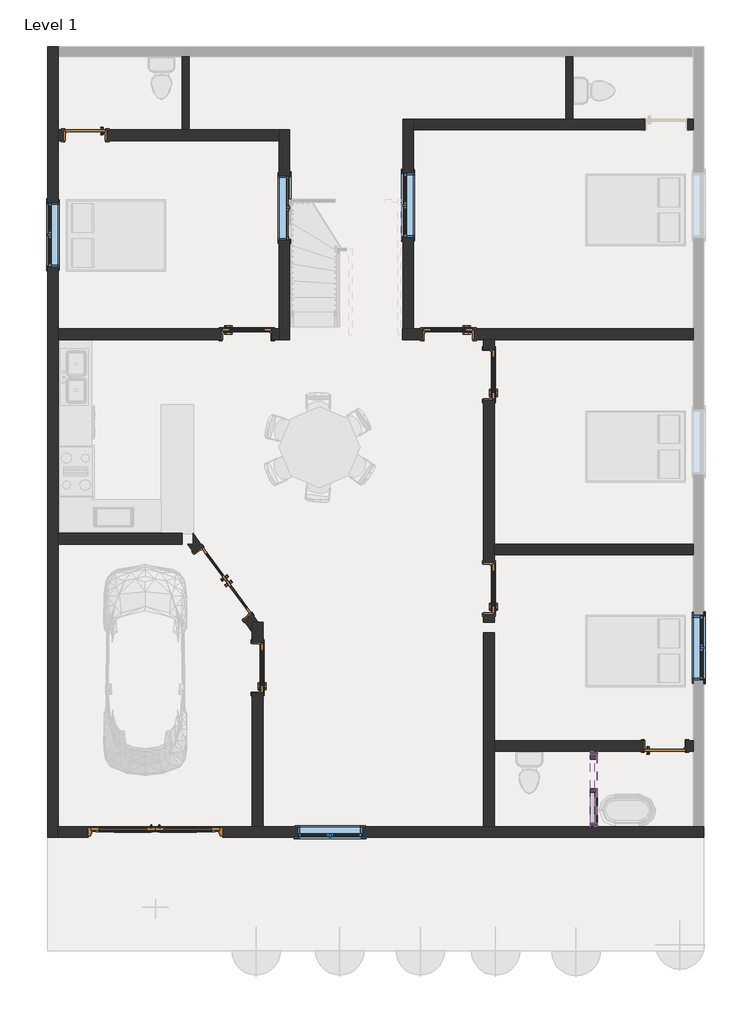
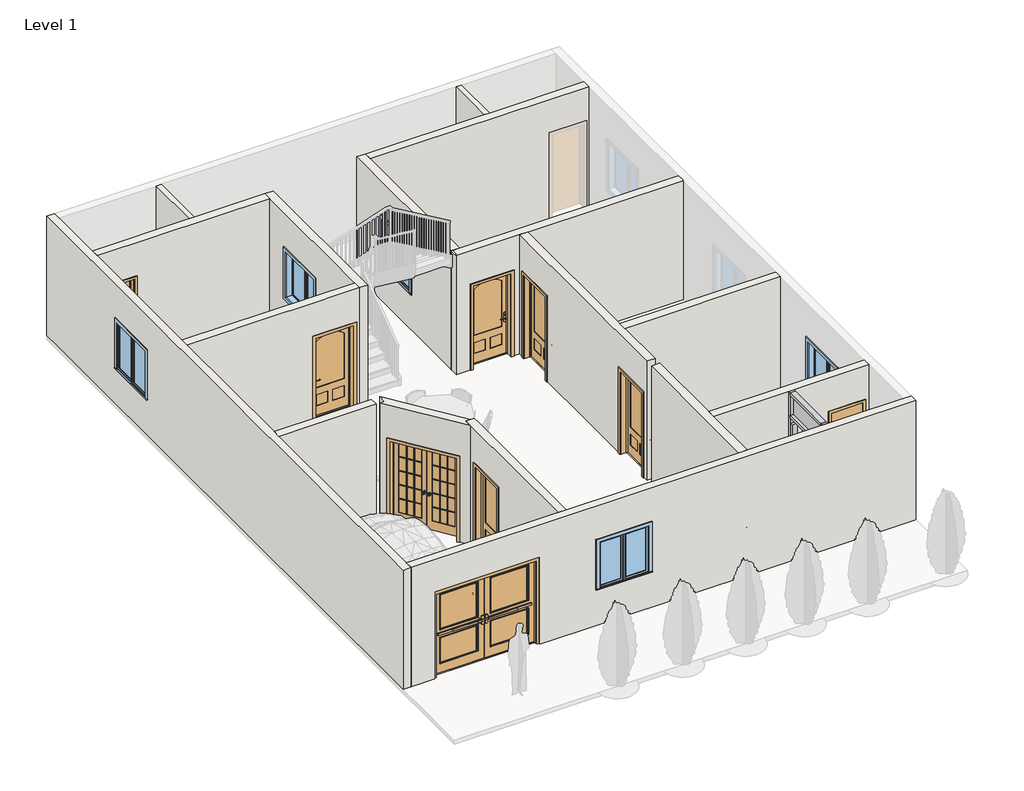
# One storey, part 1 of 3: 17 walls, 10 members, 9 doors, 5 windows, 2 plates.
"""IFC4 building model written with IfcOpenShell, lengths in millimetres."""

from ifc_helpers import new_model, si_unit, frame, origin, origin_with_axes, place, context, project, spatial, polyline, outline, extrude, faceted_brep, transform, mapped, element, save
from components import door_4a215221, door_9fdf8246, door_14451ac2, door_142f3e8c, door_1bf41894, door_15ec6cad, door_701f8457, member_ee409385, member_c8c2a2fa, member_ccee4eb0, member_cc169a76, member_860c46db, member_ba732fc4, member_623bfa76, member_547128e5, member_47bfaf8a, system_panel_glazed_bef2143c, system_panel_glazed_3ed2553b, window_0862ab64, window_d2c79e1c

model = new_model("IFC4")

# Units and contexts
model_context = context("Model", 3, world=origin())
ifc_project = project(units=[si_unit("LENGTHUNIT", "METRE", prefix="MILLI")], contexts=[model_context])

# Site, building, storey
site = spatial("IfcSite", under=ifc_project)
building = spatial("IfcBuilding", under=site)
storey = spatial("IfcBuildingStorey", under=building, Name="Level 1", Elevation=0.0)

# Doors
placement = place(None, origin())
door_shape = door_4a215221(model_context)
element("IfcDoor", 1, ObjectType="36\" x 84\"", at=placement, inside=storey, context=model_context, shape_type="MappedRepresentation", body=[
    mapped(door_shape, transform((5765.6625253, 2165.4527309, 0.0), x_axis=(0.0, -1.0, 0.0), y_axis=(1.0, 0.0, 0.0), z_axis=(0.0, 0.0, 1.0))),
])
element("IfcDoor", 2, ObjectType="36\" x 84\"", at=placement, inside=storey, context=model_context, shape_type="MappedRepresentation", body=[
    mapped(door_shape, transform((5765.6625253, -1873.1472691, 0.0), x_axis=(0.0, -1.0, 0.0), y_axis=(1.0, 0.0, 0.0), z_axis=(0.0, 0.0, 1.0))),
])
element("IfcDoor", 3, ObjectType="36\" x 84\"", at=placement, inside=storey, context=model_context, shape_type="MappedRepresentation", body=[
    mapped(door_shape, transform((4995.7250253, 2930.6277309, 0.0), x_axis=(1.0, 0.0, 0.0), y_axis=(0.0, 1.0, 0.0), z_axis=(0.0, 0.0, 1.0))),
])
element("IfcDoor", 4, ObjectType="36\" x 84\"", at=placement, inside=storey, context=model_context, shape_type="MappedRepresentation", body=[
    mapped(door_shape, transform((1392.1000253, -3371.7472691, 0.0), x_axis=(0.0, -1.0, 0.0), y_axis=(1.0, 0.0, 0.0), z_axis=(0.0, 0.0, 1.0))),
])
door_2_shape = door_9fdf8246(model_context)
element("IfcDoor", 5, ObjectType="36\" x 84\"", at=placement, inside=storey, context=model_context, shape_type="MappedRepresentation", body=[
    mapped(door_2_shape, transform((1185.7250253, 2930.6277309, 0.0), x_axis=(-1.0, 0.0, 0.0), y_axis=(0.0, -1.0, 0.0), z_axis=(0.0, 0.0, 1.0))),
])
door_3_shape = door_14451ac2(model_context)
door_4_shape = door_142f3e8c(model_context)
door_5_shape = door_1bf41894(model_context)
element("IfcDoor", 6, ObjectType="Door-Exterior-Double-Two_Lite : 96\" x 84\"", at=placement, inside=storey, context=model_context, shape_type="MappedRepresentation", body=[
    mapped(door_3_shape, transform((-541.4749747, -6476.8972691, 0.0), x_axis=(1.0, 0.0, 0.0), y_axis=(0.0, 1.0, 0.0), z_axis=(0.0, 0.0, 1.0))),
    mapped(door_4_shape, transform((-541.4749747, -6476.8972691, 0.0), x_axis=(1.0, 0.0, 0.0), y_axis=(0.0, 1.0, 0.0), z_axis=(0.0, 0.0, 1.0))),
    mapped(door_5_shape, transform((-541.4749747, -6476.8972691, 0.0), x_axis=(1.0, 0.0, 0.0), y_axis=(0.0, 1.0, 0.0), z_axis=(0.0, 0.0, 1.0))),
])
door_6_shape = door_15ec6cad(model_context)
element("IfcDoor", 7, ObjectType="Door-Interior-Double-Full Glass-Wood : 60\" x 84\"", at=placement, inside=storey, context=model_context, shape_type="MappedRepresentation", body=[
    mapped(door_6_shape, transform((739.9205393, -1775.5962656, 0.0), x_axis=(0.5914191036451608, -0.8063643369120156, 0.0), y_axis=(0.8063643369120156, 0.5914191036451608, 0.0), z_axis=(0.0, 0.0, 1.0))),
])
door_7_shape = door_701f8457(model_context)
element("IfcDoor", 8, ObjectType="Door-Interior-Single-Flush_Panel-Wood : 30\" x 84\"", at=placement, inside=storey, context=model_context, shape_type="MappedRepresentation", body=[
    mapped(door_7_shape, transform((-1867.0374747, 6689.8277309, 0.0), x_axis=(-1.0, 0.0, 0.0), y_axis=(0.0, -1.0, 0.0), z_axis=(0.0, 0.0, 1.0))),
])
element("IfcDoor", 9, ObjectType="Door-Interior-Single-Flush_Panel-Wood : 30\" x 84\"", at=placement, inside=storey, context=model_context, shape_type="MappedRepresentation", body=[
    mapped(door_7_shape, transform((9089.8875253, -4848.1222691, 0.0), x_axis=(1.0, 0.0, 0.0), y_axis=(0.0, 1.0, 0.0), z_axis=(0.0, 0.0, 1.0))),
])

# Members
member_shape = member_ee409385(model_context)
element("IfcMember", 10, ObjectType="Rectangular Mullion : 2.5\" x 5\" rectangular", at=placement, inside=storey, context=model_context, shape_type="MappedRepresentation", body=[
    mapped(member_shape, transform((7743.6875253, -6368.9472691, 0.0), x_axis=(0.0, -1.0, 0.0), y_axis=(-1.0, 0.0, 0.0), z_axis=(0.0, 0.0, -1.0))),
])
member_2_shape = member_c8c2a2fa(model_context)
element("IfcMember", 11, ObjectType="Rectangular Mullion : 2.5\" x 5\" rectangular", at=placement, inside=storey, context=model_context, shape_type="MappedRepresentation", body=[
    mapped(member_2_shape, transform((7743.6875253, -6305.4472691, 2438.4), x_axis=(0.0, 0.0, 1.0), y_axis=(-1.0, 0.0, 0.0), z_axis=(0.0, -1.0, 0.0))),
])
member_3_shape = member_ccee4eb0(model_context)
element("IfcMember", 12, ObjectType="Rectangular Mullion : 2.5\" x 5\" rectangular", at=placement, inside=storey, context=model_context, shape_type="MappedRepresentation", body=[
    mapped(member_3_shape, transform((7743.6875253, -4946.5472691, 2438.4), x_axis=(0.0, 1.0, 0.0), y_axis=(-1.0, 0.0, 0.0), z_axis=(0.0, 0.0, 1.0))),
])
member_4_shape = member_cc169a76(model_context)
element("IfcMember", 13, ObjectType="Rectangular Mullion : 2.5\" x 5\" rectangular", at=placement, inside=storey, context=model_context, shape_type="MappedRepresentation", body=[
    mapped(member_4_shape, transform((7743.6875253, -5098.9472691, 6.4344163), x_axis=(0.0, -1.0, 0.0), y_axis=(-1.0, 0.0, 0.0), z_axis=(0.0, 0.0, -1.0))),
])
member_5_shape = member_860c46db(model_context)
element("IfcMember", 14, ObjectType="Rectangular Mullion : 2.5\" x 5\" rectangular", at=placement, inside=storey, context=model_context, shape_type="MappedRepresentation", body=[
    mapped(member_5_shape, transform((7743.6875253, -5657.7472691, 2286.0), x_axis=(0.0, 1.0, 0.0), y_axis=(-1.0, 0.0, 0.0), z_axis=(0.0, 0.0, 1.0))),
])
member_6_shape = member_ba732fc4(model_context)
element("IfcMember", 15, ObjectType="Rectangular Mullion : 2.5\" x 5\" rectangular", at=placement, inside=storey, context=model_context, shape_type="MappedRepresentation", body=[
    mapped(member_6_shape, transform((7743.6875253, -5010.0472691, 6.4344163), x_axis=(0.0, 0.0, -1.0), y_axis=(-1.0, 0.0, 0.0), z_axis=(0.0, 1.0, 0.0))),
])
member_7_shape = member_623bfa76(model_context)
element("IfcMember", 16, ObjectType="Rectangular Mullion : 2.5\" x 5\" rectangular", at=placement, inside=storey, context=model_context, shape_type="MappedRepresentation", body=[
    mapped(member_7_shape, transform((7743.6875253, -5721.2472691, 0.0), x_axis=(0.0, 0.0, -1.0), y_axis=(-1.0, 0.0, 0.0), z_axis=(0.0, 1.0, 0.0))),
])
member_8_shape = member_547128e5(model_context)
element("IfcMember", 17, ObjectType="Rectangular Mullion : 2.5\" x 5\" rectangular", at=placement, inside=storey, context=model_context, shape_type="MappedRepresentation", body=[
    mapped(member_8_shape, transform((7743.6875253, -6305.4472691, 3048.0), x_axis=(0.0, 0.0, 1.0), y_axis=(-1.0, 0.0, 0.0), z_axis=(0.0, -1.0, 0.0))),
])
member_9_shape = member_47bfaf8a(model_context)
element("IfcMember", 18, ObjectType="Rectangular Mullion : 2.5\" x 5\" rectangular", at=placement, inside=storey, context=model_context, shape_type="MappedRepresentation", body=[
    mapped(member_9_shape, transform((7743.6875253, -6368.9472691, 2438.4), x_axis=(0.0, -1.0, 0.0), y_axis=(-1.0, 0.0, 0.0), z_axis=(0.0, 0.0, -1.0))),
])
element("IfcMember", 19, ObjectType="Rectangular Mullion : 2.5\" x 5\" rectangular", at=placement, inside=storey, context=model_context, shape_type="MappedRepresentation", body=[
    mapped(member_9_shape, transform((7743.6875253, -4946.5472691, 3048.0), x_axis=(0.0, 1.0, 0.0), y_axis=(-1.0, 0.0, 0.0), z_axis=(0.0, 0.0, 1.0))),
])

# Plates
system_panel_glazed_shape = system_panel_glazed_bef2143c(model_context)
element("IfcPlate", 20, ObjectType="System Panel : Glazed", at=placement, inside=storey, context=model_context, shape_type="MappedRepresentation", body=[
    mapped(system_panel_glazed_shape, transform((7743.6875253, -5657.7472691, 63.5), x_axis=(0.0, -1.0, 0.0), y_axis=(1.0, 0.0, 0.0), z_axis=(0.0, 0.0, 1.0))),
])
system_panel_glazed_2_shape = system_panel_glazed_3ed2553b(model_context)
element("IfcPlate", 21, ObjectType="System Panel : Glazed", at=placement, inside=storey, context=model_context, shape_type="MappedRepresentation", body=[
    mapped(system_panel_glazed_2_shape, transform((7743.6875253, -5657.7472691, 2470.15), x_axis=(0.0, -1.0, 0.0), y_axis=(1.0, 0.0, 0.0), z_axis=(0.0, 0.0, 1.0))),
])

# Walls
element("IfcWall", 22, at=placement, inside=storey, context=model_context, shape_type="Brep", body=[
    faceted_brep([(9821.7250253, -6368.9472691, 3048.0), (9821.7250253, -6368.9472691, 0.0), (9628.0500253, -6368.9472691, 0.0), (5864.0875253, -6368.9472691, 0.0), (5660.8875253, -6368.9472691, 0.0), (1490.5250253, -6368.9472691, 0.0), (1287.3250253, -6368.9472691, 0.0), (728.5250253, -6368.9472691, 0.0), (728.5250253, -6368.9472691, 2235.2), (-1811.4749747, -6368.9472691, 2235.2), (-1811.4749747, -6368.9472691, 0.0), (-2379.7999747, -6368.9472691, 0.0), (-2379.7999747, -6368.9472691, 3048.0), (1287.3250253, -6368.9472691, 3048.0), (1490.5250253, -6368.9472691, 3048.0), (5660.8875253, -6368.9472691, 3048.0), (5864.0875253, -6368.9472691, 3048.0), (9628.0500253, -6368.9472691, 3048.0), (2150.9250253, -6368.9472691, 2133.6), (2150.9250253, -6368.9472691, 914.4), (3370.1250253, -6368.9472691, 914.4), (3370.1250253, -6368.9472691, 2133.6), (9821.7250253, -6572.1472691, 0.0), (9821.7250253, -6572.1472691, 3048.0), (-2379.7999747, -6572.1472691, 3048.0), (-2379.7999747, -6572.1472691, 0.0), (-1811.4749747, -6572.1472691, 0.0), (-1811.4749747, -6572.1472691, 2235.2), (728.5250253, -6572.1472691, 2235.2), (728.5250253, -6572.1472691, 0.0), (2150.9250253, -6572.1472691, 2133.6), (3370.1250253, -6572.1472691, 2133.6), (3370.1250253, -6572.1472691, 914.4), (2150.9250253, -6572.1472691, 914.4)], [[[0, 1, 2, 3, 4, 5, 6, 7, 8, 9, 10, 11, 12, 13, 14, 15, 16, 17], [18, 19, 20, 21]], [[22, 23, 24, 25, 26, 27, 28, 29], [30, 31, 32, 33]], [[1, 22, 29, 7, 6, 5, 4, 3, 2]], [[25, 11, 10, 26]], [[1, 0, 23, 22]], [[12, 11, 25, 24]], [[28, 8, 7, 29]], [[8, 28, 27, 9]], [[9, 27, 26, 10]], [[19, 18, 30, 33]], [[20, 19, 33, 32]], [[21, 20, 32, 31]], [[18, 21, 31, 30]], [[0, 17, 16, 15, 14, 13, 12, 24, 23]]]),
])
element("IfcWall", 23, at=placement, inside=storey, context=model_context, shape_type="Brep", body=[
    faceted_brep([(1795.3250253, 6788.2527309, 0.0), (1795.3250253, 6585.0527309, 0.0), (1795.3250253, 3029.0527309, 0.0), (1795.3250253, 2825.8527309, 0.0), (1795.3250253, 2825.8527309, 3048.0), (1795.3250253, 3029.0527309, 3048.0), (1795.3250253, 6585.0527309, 3048.0), (1795.3250253, 6788.2527309, 3048.0), (1795.3250253, 4705.4527309, 2133.6), (1795.3250253, 4705.4527309, 914.4), (1795.3250253, 5924.6527309, 914.4), (1795.3250253, 5924.6527309, 2133.6), (1998.5250253, 6788.2527309, 0.0), (1998.5250253, 6788.2527309, 3048.0), (1998.5250253, 2825.8527309, 3048.0), (1998.5250253, 2825.8527309, 0.0), (1998.5250253, 4705.4527309, 2133.6), (1998.5250253, 5924.6527309, 2133.6), (1998.5250253, 5924.6527309, 914.4), (1998.5250253, 4705.4527309, 914.4)], [[[0, 1, 2, 3, 4, 5, 6, 7], [8, 9, 10, 11]], [[12, 13, 14, 15], [16, 17, 18, 19]], [[3, 2, 1, 0, 12, 15]], [[4, 3, 15, 14]], [[0, 7, 13, 12]], [[9, 8, 16, 19]], [[10, 9, 19, 18]], [[11, 10, 18, 17]], [[8, 11, 17, 16]], [[7, 6, 5, 4, 14, 13]]]),
])
element("IfcWall", 24, at=placement, inside=storey, context=model_context, shape_type="Brep", body=[
    faceted_brep([(1795.3250253, 3029.0527309, 3048.0), (1795.3250253, 3029.0527309, 0.0), (1668.3250253, 3029.0527309, 0.0), (1668.3250253, 3029.0527309, 2159.0), (703.1250253, 3029.0527309, 2159.0), (703.1250253, 3029.0527309, 0.0), (-2379.7999747, 3029.0527309, 0.0), (-2379.7999747, 3029.0527309, 3048.0), (1795.3250253, 2825.8527309, 0.0), (1795.3250253, 2825.8527309, 3048.0), (169.7250253, 2825.8527309, 3048.0), (-33.4749747, 2825.8527309, 3048.0), (-2379.7999747, 2825.8527309, 3048.0), (-2379.7999747, 2825.8527309, 0.0), (-33.4749747, 2825.8527309, 0.0), (169.7250253, 2825.8527309, 0.0), (703.1250253, 2825.8527309, 0.0), (703.1250253, 2825.8527309, 2159.0), (1668.3250253, 2825.8527309, 2159.0), (1668.3250253, 2825.8527309, 0.0)], [[[0, 1, 2, 3, 4, 5, 6, 7]], [[8, 9, 10, 11, 12, 13, 14, 15, 16, 17, 18, 19]], [[1, 8, 19, 2]], [[13, 6, 5, 16, 15, 14]], [[1, 0, 9, 8]], [[7, 6, 13, 12]], [[4, 17, 16, 5]], [[17, 4, 3, 18]], [[18, 3, 2, 19]], [[0, 7, 12, 11, 10, 9]]]),
])
element("IfcWall", 25, at=placement, inside=storey, context=model_context, shape_type="Brep", body=[
    faceted_brep([(4132.1250253, 2825.8527309, 3048.0), (4132.1250253, 2825.8527309, 0.0), (4513.1250253, 2825.8527309, 0.0), (4513.1250253, 2825.8527309, 2159.0), (5478.3250253, 2825.8527309, 2159.0), (5478.3250253, 2825.8527309, 0.0), (5660.8875253, 2825.8527309, 0.0), (5864.0875253, 2825.8527309, 0.0), (9628.0500253, 2825.8527309, 0.0), (9628.0500253, 2825.8527309, 3048.0), (5864.0875253, 2825.8527309, 3048.0), (5660.8875253, 2825.8527309, 3048.0), (4132.1250253, 3029.0527309, 0.0), (4132.1250253, 3029.0527309, 3048.0), (4136.9635307, 3029.0527309, 3048.0), (4164.6571636, 3029.0527309, 3048.0), (4340.1635307, 3029.0527309, 3048.0), (9628.0500253, 3029.0527309, 3048.0), (9628.0500253, 3029.0527309, 0.0), (5478.3250253, 3029.0527309, 0.0), (5478.3250253, 3029.0527309, 2159.0), (4513.1250253, 3029.0527309, 2159.0), (4513.1250253, 3029.0527309, 0.0), (4340.1635307, 3029.0527309, 0.0), (4136.9635307, 3029.0527309, 0.0), (4132.1250253, 2881.9427876, 3048.0), (9628.0500253, 2881.9427876, 3048.0), (4167.6535874, 2881.9427876, 3048.0)], [[[0, 1, 2, 3, 4, 5, 6, 7, 8, 9, 10, 11]], [[12, 13, 14, 15, 16, 17, 18, 19, 20, 21, 22, 23, 24]], [[1, 12, 24, 23, 22, 2]], [[18, 8, 7, 6, 5, 19]], [[1, 0, 25, 13, 12]], [[9, 8, 18, 17, 26]], [[4, 20, 19, 5]], [[20, 4, 3, 21]], [[21, 3, 2, 22]], [[13, 25, 27, 15, 14]], [[25, 0, 11, 10, 9, 26, 17, 16, 15, 27]]]),
])
element("IfcWall", 26, at=placement, inside=storey, context=model_context, shape_type="Brep", body=[
    faceted_brep([(1490.5250253, -6368.9472691, 3048.0), (1490.5250253, -6368.9472691, 0.0), (1490.5250253, -3854.3472691, 0.0), (1490.5250253, -3854.3472691, 2159.0), (1490.5250253, -2889.1472691, 2159.0), (1490.5250253, -2889.1472691, 0.0), (1490.5250253, -2711.3472691, 0.0), (1490.5250253, -2508.1472691, 0.0), (1490.5250253, -2508.1472691, 3048.0), (1490.5250253, -2711.3472691, 3048.0), (1287.3250253, -6368.9472691, 0.0), (1287.3250253, -6368.9472691, 3048.0), (1287.3250253, -2699.1079548, 3048.0), (1287.3250253, -2508.1472691, 3048.0), (1287.3250253, -2508.1472691, 0.0), (1287.3250253, -2699.1079548, 0.0), (1287.3250253, -2889.1472691, 0.0), (1287.3250253, -2889.1472691, 2159.0), (1287.3250253, -3854.3472691, 2159.0), (1287.3250253, -3854.3472691, 0.0), (1399.2622704, -2508.1472691, 0.0), (1399.2622704, -2508.1472691, 3048.0)], [[[0, 1, 2, 3, 4, 5, 6, 7, 8, 9]], [[10, 11, 12, 13, 14, 15, 16, 17, 18, 19]], [[1, 10, 19, 2]], [[14, 20, 7, 6, 5, 16, 15]], [[1, 0, 11, 10]], [[8, 7, 20, 14, 13, 21]], [[18, 3, 2, 19]], [[3, 18, 17, 4]], [[4, 17, 16, 5]], [[0, 9, 8, 21, 13, 12, 11]]]),
])
element("IfcWall", 27, at=placement, inside=storey, context=model_context, shape_type="Brep", body=[
    faceted_brep([(5660.8875253, -2711.3472691, 0.0), (5660.8875253, -6368.9472691, 0.0), (5660.8875253, -6368.9472691, 3048.0), (5660.8875253, -2711.3472691, 3048.0), (5864.0875253, -2711.3472691, 0.0), (5864.0875253, -2711.3472691, 3048.0), (5864.0875253, -4743.3472691, 3048.0), (5864.0875253, -4946.5472691, 3048.0), (5864.0875253, -6368.9472691, 3048.0), (5864.0875253, -6368.9472691, 0.0), (5864.0875253, -4946.5472691, 0.0), (5864.0875253, -4743.3472691, 0.0)], [[[0, 1, 2, 3]], [[4, 5, 6, 7, 8, 9, 10, 11]], [[1, 0, 4, 11, 10, 9]], [[0, 3, 5, 4]], [[2, 1, 9, 8]], [[3, 2, 8, 7, 6, 5]]]),
])
element("IfcWall", 28, at=placement, inside=storey, context=model_context, shape_type="SweptSolid", body=[
    extrude(outline(polyline([(0.0, 9628.0500253), (3048.0, 9628.0500253), (3048.0, 5864.0875253), (0.0, 5864.0875253), (0.0, 8683.4875253), (2159.0, 8683.4875253), (2159.0, 9496.2875253), (0.0, 9496.2875253), (0.0, 9628.0500253)])), frame((0.0, -4946.5472691, 0.0), z_axis=(0.0, 1.0, 0.0), x_axis=(0.0, 0.0, 1.0)), (0.0, 0.0, 1.0), 203.2),
])
element("IfcWall", 29, at=placement, inside=storey, context=model_context, shape_type="Brep", body=[
    faceted_brep([(5864.0875253, -2508.1472691, 3048.0), (5864.0875253, -2508.1472691, 0.0), (5864.0875253, -2355.7472691, 0.0), (5864.0875253, -2355.7472691, 2159.0), (5864.0875253, -1390.5472691, 2159.0), (5864.0875253, -1390.5472691, 0.0), (5864.0875253, -1238.1472691, 0.0), (5864.0875253, -1034.9472691, 0.0), (5864.0875253, 1682.8527309, 0.0), (5864.0875253, 1682.8527309, 2159.0), (5864.0875253, 2648.0527309, 2159.0), (5864.0875253, 2648.0527309, 0.0), (5864.0875253, 2825.8527309, 0.0), (5864.0875253, 2825.8527309, 3048.0), (5864.0875253, -1034.9472691, 3048.0), (5864.0875253, -1238.1472691, 3048.0), (5660.8875253, -2508.1472691, 0.0), (5660.8875253, -2508.1472691, 3048.0), (5660.8875253, 2825.8527309, 3048.0), (5660.8875253, 2825.8527309, 0.0), (5660.8875253, 2648.0527309, 0.0), (5660.8875253, 2648.0527309, 2159.0), (5660.8875253, 1682.8527309, 2159.0), (5660.8875253, 1682.8527309, 0.0), (5660.8875253, -1390.5472691, 0.0), (5660.8875253, -1390.5472691, 2159.0), (5660.8875253, -2355.7472691, 2159.0), (5660.8875253, -2355.7472691, 0.0)], [[[0, 1, 2, 3, 4, 5, 6, 7, 8, 9, 10, 11, 12, 13, 14, 15]], [[16, 17, 18, 19, 20, 21, 22, 23, 24, 25, 26, 27]], [[1, 16, 27, 2]], [[19, 12, 11, 20]], [[23, 8, 7, 6, 5, 24]], [[1, 0, 17, 16]], [[13, 12, 19, 18]], [[22, 9, 8, 23]], [[9, 22, 21, 10]], [[10, 21, 20, 11]], [[26, 3, 2, 27]], [[3, 26, 25, 4]], [[4, 25, 24, 5]], [[0, 15, 14, 13, 18, 17]]]),
])
element("IfcWall", 30, at=placement, inside=storey, context=model_context, shape_type="SweptSolid", body=[
    extrude(outline(polyline([(5864.0875253, -1034.9472691), (9628.0500253, -1034.9472691), (9628.0500253, -1238.1472691), (5864.0875253, -1238.1472691), (5864.0875253, -1034.9472691)])), origin_with_axes(), (0.0, 0.0, 1.0), 3048.0),
])
element("IfcWall", 31, at=placement, inside=storey, context=model_context, shape_type="Brep", body=[
    faceted_brep([(1287.3250253, -2699.1079548, 0.0), (1287.3250253, -2699.1079548, 3048.0), (66.7645714, -1034.9472691, 3048.0), (66.7645714, -1034.9472691, 0.0), (189.7503136, -1202.6309233, 0.0), (189.7503136, -1202.6309233, 2159.0), (1121.1171181, -2472.4934811, 2159.0), (1121.1171181, -2472.4934811, 0.0), (1399.2622704, -2508.1472691, 3048.0), (1399.2622704, -2508.1472691, 0.0), (1284.9703513, -2352.3171192, 0.0), (1284.9703513, -2352.3171192, 2159.0), (353.6035469, -1082.4545614, 2159.0), (353.6035469, -1082.4545614, 0.0), (169.7250253, -831.7472691, 0.0), (169.7250253, -831.7472691, 3048.0), (1287.3250253, -2508.1472691, 0.0), (169.7250253, -1034.9472691, 0.0), (1287.3250253, -2508.1472691, 3048.0), (169.7250253, -1034.9472691, 3048.0)], [[[0, 1, 2, 3, 4, 5, 6, 7]], [[8, 9, 10, 11, 12, 13, 14, 15]], [[9, 16, 0, 7, 10]], [[3, 17, 14, 13, 4]], [[1, 0, 16, 18]], [[9, 8, 18, 16]], [[6, 11, 10, 7]], [[11, 6, 5, 12]], [[12, 5, 4, 13]], [[17, 3, 2, 19]], [[14, 17, 19, 15]], [[2, 1, 18, 8, 15, 19]]]),
])
element("IfcWall", 32, at=placement, inside=storey, context=model_context, shape_type="Brep", body=[
    faceted_brep([(4136.9635307, 6991.4527309, 0.0), (4136.9635307, 3029.0527309, 0.0), (4136.9635307, 3029.0527309, 3048.0), (4136.9635307, 6991.4527309, 3048.0), (4136.9635307, 5975.4527309, 2133.6), (4136.9635307, 4756.2527309, 2133.6), (4136.9635307, 4756.2527309, 914.4), (4136.9635307, 5975.4527309, 914.4), (4340.1635307, 6991.4527309, 0.0), (4340.1635307, 6991.4527309, 3048.0), (4340.1635307, 6788.2527309, 3048.0), (4340.1635307, 3029.0527309, 3048.0), (4340.1635307, 3029.0527309, 0.0), (4340.1635307, 6788.2527309, 0.0), (4340.1635307, 5975.4527309, 2133.6), (4340.1635307, 5975.4527309, 914.4), (4340.1635307, 4756.2527309, 914.4), (4340.1635307, 4756.2527309, 2133.6)], [[[0, 1, 2, 3], [4, 5, 6, 7]], [[8, 9, 10, 11, 12, 13], [14, 15, 16, 17]], [[1, 0, 8, 13, 12]], [[3, 2, 11, 10, 9]], [[2, 1, 12, 11]], [[0, 3, 9, 8]], [[15, 14, 4, 7]], [[16, 15, 7, 6]], [[17, 16, 6, 5]], [[14, 17, 5, 4]]]),
])
element("IfcWall", 33, ObjectType="Generic - 5\"", at=placement, inside=storey, context=model_context, shape_type="SweptSolid", body=[
    extrude(outline(polyline([(-33.4749747, 6788.2527309), (-33.4749747, 8169.3777309), (93.5250253, 8169.3777309), (93.5250253, 6788.2527309), (-33.4749747, 6788.2527309)])), origin_with_axes(), (0.0, 0.0, 1.0), 3048.0),
])
element("IfcWall", 34, ObjectType="Generic - 5\"", at=placement, inside=storey, context=model_context, shape_type="SweptSolid", body=[
    extrude(outline(polyline([(7218.2250253, 6991.4527309), (7218.2250253, 8169.3777309), (7345.2250253, 8169.3777309), (7345.2250253, 6991.4527309), (7218.2250253, 6991.4527309)])), origin_with_axes(), (0.0, 0.0, 1.0), 3048.0),
])
element("IfcWall", 35, ObjectType="Generic - 8\"", at=placement, inside=storey, context=model_context, shape_type="SweptSolid", body=[
    extrude(outline(polyline([(-2379.7999747, -831.7472691), (-33.4749747, -831.7472691), (-33.4749747, -1034.9472691), (-2379.7999747, -1034.9472691), (-2379.7999747, -831.7472691)])), origin_with_axes(), (0.0, 0.0, 1.0), 3048.0),
])
element("IfcWall", 36, ObjectType="Generic - 8\"", at=placement, inside=storey, context=model_context, shape_type="Brep", body=[
    faceted_brep([(1795.3250253, 6788.2527309, 3048.0), (1795.3250253, 6788.2527309, 0.0), (93.5250253, 6788.2527309, 0.0), (-33.4749747, 6788.2527309, 0.0), (-1460.6374747, 6788.2527309, 0.0), (-1460.6374747, 6788.2527309, 2159.0), (-2273.4374747, 6788.2527309, 2159.0), (-2273.4374747, 6788.2527309, 0.0), (-2379.7999747, 6788.2527309, 0.0), (-2379.7999747, 6788.2527309, 3048.0), (-33.4749747, 6788.2527309, 3048.0), (93.5250253, 6788.2527309, 3048.0), (1795.3250253, 6585.0527309, 0.0), (1795.3250253, 6585.0527309, 3048.0), (-2379.7999747, 6585.0527309, 3048.0), (-2379.7999747, 6585.0527309, 0.0), (-2273.4374747, 6585.0527309, 0.0), (-2273.4374747, 6585.0527309, 2159.0), (-1460.6374747, 6585.0527309, 2159.0), (-1460.6374747, 6585.0527309, 0.0)], [[[0, 1, 2, 3, 4, 5, 6, 7, 8, 9, 10, 11]], [[12, 13, 14, 15, 16, 17, 18, 19]], [[1, 12, 19, 4, 3, 2]], [[15, 8, 7, 16]], [[1, 0, 13, 12]], [[9, 8, 15, 14]], [[6, 17, 16, 7]], [[17, 6, 5, 18]], [[18, 5, 4, 19]], [[0, 11, 10, 9, 14, 13]]]),
])
element("IfcWall", 37, ObjectType="Generic - 8\"", at=placement, inside=storey, context=model_context, shape_type="Brep", body=[
    faceted_brep([(4340.1635307, 6788.2527309, 3048.0), (4340.1635307, 6788.2527309, 0.0), (8708.8875253, 6788.2527309, 0.0), (8708.8875253, 6788.2527309, 2159.0), (9521.6875253, 6788.2527309, 2159.0), (9521.6875253, 6788.2527309, 0.0), (9628.0500253, 6788.2527309, 0.0), (9628.0500253, 6788.2527309, 3048.0), (4340.1635307, 6991.4527309, 0.0), (4340.1635307, 6991.4527309, 3048.0), (7218.2250253, 6991.4527309, 3048.0), (7345.2250253, 6991.4527309, 3048.0), (9628.0500253, 6991.4527309, 3048.0), (9628.0500253, 6991.4527309, 0.0), (9521.6875253, 6991.4527309, 0.0), (9521.6875253, 6991.4527309, 2159.0), (8708.8875253, 6991.4527309, 2159.0), (8708.8875253, 6991.4527309, 0.0), (7345.2250253, 6991.4527309, 0.0), (7218.2250253, 6991.4527309, 0.0)], [[[0, 1, 2, 3, 4, 5, 6, 7]], [[8, 9, 10, 11, 12, 13, 14, 15, 16, 17, 18, 19]], [[1, 8, 19, 18, 17, 2]], [[13, 6, 5, 14]], [[1, 0, 9, 8]], [[7, 6, 13, 12]], [[4, 15, 14, 5]], [[15, 4, 3, 16]], [[16, 3, 2, 17]], [[0, 7, 12, 11, 10, 9]]]),
])
element("IfcWall", 38, ObjectType="a", at=placement, inside=storey, context=model_context, shape_type="Brep", body=[
    faceted_brep([(-2379.7999747, -6572.1472691, 0.0), (-2379.7999747, -6368.9472691, 0.0), (-2379.7999747, -1034.9472691, 0.0), (-2379.7999747, -831.7472691, 0.0), (-2379.7999747, 2825.8527309, 0.0), (-2379.7999747, 3029.0527309, 0.0), (-2379.7999747, 6585.0527309, 0.0), (-2379.7999747, 6788.2527309, 0.0), (-2379.7999747, 8169.3777309, 0.0), (-2379.7999747, 8363.0527309, 0.0), (-2379.7999747, 8363.0527309, 3048.0), (-2379.7999747, 8169.3777309, 3048.0), (-2379.7999747, 6788.2527309, 3048.0), (-2379.7999747, 6585.0527309, 3048.0), (-2379.7999747, 3029.0527309, 3048.0), (-2379.7999747, 2825.8527309, 3048.0), (-2379.7999747, -831.7472691, 3048.0), (-2379.7999747, -1034.9472691, 3048.0), (-2379.7999747, -6368.9472691, 3048.0), (-2379.7999747, -6572.1472691, 3048.0), (-2379.7999747, 5416.6527309, 2133.6), (-2379.7999747, 5416.6527309, 914.4), (-2379.7999747, 4197.4527309, 914.4), (-2379.7999747, 4197.4527309, 2133.6), (-2573.4749747, -6572.1472691, 0.0), (-2573.4749747, -6572.1472691, 3048.0), (-2573.4749747, 8363.0527309, 3048.0), (-2573.4749747, 8363.0527309, 0.0), (-2573.4749747, 5416.6527309, 2133.6), (-2573.4749747, 4197.4527309, 2133.6), (-2573.4749747, 4197.4527309, 914.4), (-2573.4749747, 5416.6527309, 914.4)], [[[0, 1, 2, 3, 4, 5, 6, 7, 8, 9, 10, 11, 12, 13, 14, 15, 16, 17, 18, 19], [20, 21, 22, 23]], [[24, 25, 26, 27], [28, 29, 30, 31]], [[0, 19, 25, 24]], [[10, 9, 27, 26]], [[21, 20, 28, 31]], [[22, 21, 31, 30]], [[23, 22, 30, 29]], [[20, 23, 29, 28]], [[19, 18, 17, 16, 15, 14, 13, 12, 11, 10, 26, 25]], [[9, 8, 7, 6, 5, 4, 3, 2, 1, 0, 24, 27]]]),
])

# Windows
window_shape = window_0862ab64(model_context)
element("IfcWindow", 39, ObjectType="Casement Dbl with Trim : 48\" x 48\"", at=placement, inside=storey, context=model_context, shape_type="MappedRepresentation", body=[
    mapped(window_shape, transform((2760.5250253, -6451.4972691, 0.0), x_axis=(-1.0, 0.0, 0.0), y_axis=(0.0, -1.0, 0.0), z_axis=(0.0, 0.0, 1.0))),
])
window_2_shape = window_d2c79e1c(model_context)
element("IfcWindow", 40, ObjectType="Casement Dbl with Trim : 48\" x 48\"", at=placement, inside=storey, context=model_context, shape_type="MappedRepresentation", body=[
    mapped(window_2_shape, transform((9705.8375253, -2990.7472691, 0.0), x_axis=(0.0, -1.0, 0.0), y_axis=(1.0, 0.0, 0.0), z_axis=(0.0, 0.0, 1.0))),
])
element("IfcWindow", 41, ObjectType="Casement Dbl with Trim : 48\" x 48\"", at=placement, inside=storey, context=model_context, shape_type="MappedRepresentation", body=[
    mapped(window_shape, transform((1877.8750253, 5315.0527309, 0.0), x_axis=(0.0, -1.0, 0.0), y_axis=(1.0, 0.0, 0.0), z_axis=(0.0, 0.0, 1.0))),
])
element("IfcWindow", 42, ObjectType="Casement Dbl with Trim : 48\" x 48\"", at=placement, inside=storey, context=model_context, shape_type="MappedRepresentation", body=[
    mapped(window_shape, transform((4257.6135307, 5365.8527309, 0.0), x_axis=(0.0, 1.0, 0.0), y_axis=(-1.0, 0.0, 0.0), z_axis=(0.0, 0.0, 1.0))),
])
element("IfcWindow", 43, ObjectType="Casement Dbl with Trim : 48\" x 48\"", at=placement, inside=storey, context=model_context, shape_type="MappedRepresentation", body=[
    mapped(window_2_shape, transform((-2457.5874747, 4807.0527309, 0.0), x_axis=(0.0, 1.0, 0.0), y_axis=(-1.0, 0.0, 0.0), z_axis=(0.0, 0.0, 1.0))),
])

save(model, "model.ifc")

# Revit data of these elements
# Type "36\" x 84\""
#   Type Mark = "11"
#   Assembly Code = "B2030100"
#   Analytic Construction = "French door, wood frame with single glass"
#   Threshold Offset [instance default] = 0' - 0 1/2"
#   Thickness = 0' - 1 3/8"
#   Thermal Resistance (R) = 1.0696 (h·ft²·°F)/BTU
#   Swing Angle [instance default] = 90.00°
#   Stiles = 0' - 4 3/4"
#   Rough Width = 3' - 2"
#   Rough Height = 7' - 1"
#   Radius = 1' - 8.05625"
#   Lock Rail = 0' - 7 1/8"
#   Height = 7' - 0"
#   Width = 3' - 0"
#   Heat Transfer Coefficient (U) = 0.9350 BTU/(h·ft²·°F)
#   Door Offset [instance default] = 0' - 0"
#   Bottom Rail = 0' - 9 1/2"
#   Threshold [instance default] = yes
#   Function = 1
#   Exterior Trim [instance default] = yes
#   Trim Material = Cherry
#   Threshold Material = Cherry
#   Panel Material = Cherry
#   Glazing = Glass
#   Frame Material = Cherry
#   Door Handle Material = Aluminum
#   Visual Light Transmittance = 0
#   Solar Heat Gain Coefficient = 0
#   Wall Closure = (empty or 0)
#   Construction Type = (empty or 0)
# Type "Door-Exterior-Double-Two_Lite : 96\" x 84\""
#   Type Mark = "8"
#   Assembly Code = "B2030100"
#   Analytic Construction = "Metal frame, double glass door"
#   Top Rail = 0' - 4 5/8"
#   Threshold Length [instance default] = 8' - 4"
#   Threshold Offset [instance default] = 0' - 0 1/2"
#   Thickness = 0' - 1 3/4"
#   Thermal Resistance (R) = 1.3794 (h·ft²·°F)/BTU
#   Swing Angle [instance default] = 90.00°
#   Strike Height = 3' - 4"
#   Stiles = 0' - 6"
#   SinglePanelWidth = 4' - 0"
#   Rough Width [instance default] = 8' - 4"
#   Rough Height [instance default] = 7' - 4"
#   MFOpeningHeight [instance default] = 0' - 4"
#   MFOpeningWidth [instance default] = 0' - 4"
#   Lock Rail = 0' - 8"
#   Inset Calculate [instance default] = 0' - 4"
#   Masonry Inset [instance default] = 0' - 1"
#   Height = 7' - 0"
#   Width = 8' - 0"
#   Heat Transfer Coefficient (U) = 0.7250 BTU/(h·ft²·°F)
#   Glass Thickness = 0' - 0 3/4"
#   Masonry Frame Depth = 0' - 5 3/4"
#   Bottom Rail = 0' - 10"
#   Threshold [instance default] = yes
#   Masonry Frame [instance default] = yes
#   Wall Closure = 3
#   Function = 1
#   Dry Wall Frame [instance default] = no
#   Threshold Material = none
#   Panic Bar Material = Metal - Stainless Steel
#   Panel Material = Metal - Painted - Grey
#   Glass Stop Material = Metal - Painted - Grey
#   Frame Material = Metal - Painted - Grey
#   Exterior Pull Material = Metal - Stainless Steel
#   Visual Light Transmittance = 0
#   Solar Heat Gain Coefficient = 0
# Type "Door-Interior-Double-Full Glass-Wood : 60\" x 84\""
#   Type Mark = "9"
#   Assembly Code = "C1020300"
#   Analytic Construction = "French door, wood frame with single glass"
#   Top Rail = 0' - 4 11/16"
#   Thickness = 0' - 1 3/8"
#   Thermal Resistance (R) = 1.0696 (h·ft²·°F)/BTU
#   Swing Angle [instance default] = 90.00°
#   Stiles = 0' - 4 3/4"
#   Rough Width = 5' - 2"
#   Rough Height = 7' - 1"
#   Panel Width = 2' - 6"
#   Height = 7' - 0"
#   Width = 5' - 0"
#   Heat Transfer Coefficient (U) = 0.9350 BTU/(h·ft²·°F)
#   Bottom Rail = 0' - 9 1/8"
#   Show Grill [instance default] = yes
#   Trim Material = Cherry
#   Panel Material = Cherry
#   Frame Material = Cherry
#   Door Handle Material = Aluminum
#   Visual Light Transmittance = 0
#   Solar Heat Gain Coefficient = 0
#   Wall Closure = (empty or 0)
#   Function = (empty or 0)
# Type "Door-Interior-Single-Flush_Panel-Wood : 30\" x 84\""
#   Type Mark = "12"
#   Assembly Code = "C1020300"
#   Analytic Construction = "Wooden"
#   Thickness = 0' - 1 3/8"
#   Thermal Resistance (R) = 2.5876 (h·ft²·°F)/BTU
#   Swing Angle [instance default] = 90.00°
#   Rough Width = 2' - 8"
#   Rough Height = 7' - 1"
#   Height = 7' - 0"
#   Width = 2' - 6"
#   Heat Transfer Coefficient (U) = 0.3865 BTU/(h·ft²·°F)
#   Trim Material = Cherry
#   Panel Material = Cherry
#   Frame Material = Cherry
#   Door Handle Material = Aluminum
#   Visual Light Transmittance = 0
#   Solar Heat Gain Coefficient = 0
#   Wall Closure = (empty or 0)
#   Function = (empty or 0)
# Type "Rectangular Mullion : 2.5\" x 5\" rectangular"
#   built-in parameter 1007304 = 0.416667 (stored number, unit not read)
#   built-in parameter 1007301 = 0.104167 (stored number, unit not read)
#   built-in parameter 1007300 = 0.104167 (stored number, unit not read)
# Type "System Panel : Glazed"
#   Construction Type Id = "GSP4R"
#   Analytic Construction = "1/8 in Pilkington single glazing"
#   Visual Light Transmittance = 0.9
#   Solar Heat Gain Coefficient = 0.86
#   Heat Transfer Coefficient (U) = 1.18115 BTU/(h·ft²·°F)
# Type
#   Assembly Code = "B2010"
#   Layers, outside or top first: 0' - 8" "Carpet (1)" (function 1)
# Type
#   Assembly Code = "B2010"
#   Layers, outside or top first: 0' - 8" "Softwood, Lumber" (function 1)
# Type "Generic - 5\""
#   Assembly Code = "B2010"
#   Layers, outside or top first: 0' - 5" "Metal Door - Red" (function 1)
# Type "Generic - 8\""
#   Assembly Code = "B2010"
#   Layers, outside or top first: 0' - 8" "Softwood, Lumber" (function 1)
# Type "a"
#   Assembly Code = "B2010"
#   Layers, outside or top first: 0' - 7 5/8" "Brick, Common" (function 1)
# Type "Casement Dbl with Trim : 48\" x 48\""
#   Type Mark = "10"
#   Construction Type Id = "GSP4R"
#   Assembly Code = "B2020100"
#   Analytic Construction = "1/8 in Pilkington single glazing"
#   Visual Light Transmittance = 0.9
#   Solar Heat Gain Coefficient = 0.78
#   Heat Transfer Coefficient (U) = 0.6496 BTU/(h·ft²·°F)
#   Height = 4' - 0"
#   Default Sill Height = 3' - 0"
#   Trim Projection - Ext. = 0' - 0 1/2"
#   Trim Projection - Int. = 0' - 0 3/4"
#   Trim Width - Exterior = 0' - 3 1/2"
#   Trim Width - Interior = 0' - 3 1/2"
#   Width = 4' - 0"
#   Window Inset = 0' - 0 3/4"
#   Define Thermal Properties by = 1
#   Glass Pane Material = Glass
#   Sash Material = Sash
#   Trim Exterior Material = Trim
#   Trim Interior Material = Trim
#   Wall Closure = (empty or 0)
# Elements 1, 2, 3, 4, 5 (IfcDoor, "36\" x 84\"")
#   Threshold Offset = 0' - 0 1/2"
#   Swing Angle = 90.00°
#   Door Offset = 0' - 0"
#   Threshold = yes
#   Exterior Trim = yes
#   Phase Created = New Construction
#   Materials on its faces: "Cherry", "Aluminum", "Glass"
# Element 6 (IfcDoor, "Door-Exterior-Double-Two_Lite : 96\" x 84\"")
#   Threshold Offset = 0' - 0 1/2"
#   Threshold Length = 8' - 4"
#   Swing Angle = 90.00°
#   Rough Width = 8' - 4"
#   Rough Height = 7' - 4"
#   Masonry Inset = 0' - 1"
#   MFOpeningWidth = 0' - 4"
#   MFOpeningHeight = 0' - 4"
#   Inset Calculate = 0' - 4"
#   Threshold = yes
#   Masonry Frame = yes
#   Dry Wall Frame = no
#   Phase Created = New Construction
#   Materials on its faces: "Metal - Painted - Grey", "Metal - Stainless Steel", "Glass"
# Element 7 (IfcDoor, "Door-Interior-Double-Full Glass-Wood : 60\" x 84\"")
#   Swing Angle = 90.00°
#   Show Grill = yes
#   Phase Created = New Construction
#   Materials on its faces: "Cherry", "Aluminum", "Glass"
# Elements 8, 9 (IfcDoor, "Door-Interior-Single-Flush_Panel-Wood : 30\" x 84\"")
#   Swing Angle = 90.00°
#   Phase Created = New Construction
#   Materials on its faces: "Cherry", "Aluminum"
# Elements 10, 11, 12, 13, 14, 15, 16, 17, 18, 19 (IfcMember, "Rectangular Mullion : 2.5\" x 5\" rectangular")
#   Phase Created = New Construction
#   Materials on its faces: "Aluminum"
# Elements 20, 21 (IfcPlate, "System Panel : Glazed")
#   Phase Created = New Construction
#   Materials on its faces: "Glass"
# Element 22 (IfcWall)
#   Top Offset = 0' - 0"
#   Base Offset = 0' - 0"
#   Unconnected Height = 10' - 0"
#   wall height = 10' - 0"
#   Phase Created = New Construction
#   Base Constraint = Level 1
#   Materials on its faces: "Carpet (1)", "Concrete Masonry Units"
# Elements 23, 24, 25, 26, 27, 28, 29, 30, 31, 32 (IfcWall)
#   Top Offset = 0' - 0"
#   Base Offset = 0' - 0"
#   Unconnected Height = 10' - 0"
#   wall height = 10' - 0"
#   Phase Created = New Construction
#   Base Constraint = Level 1
#   Materials on its faces: "Softwood, Lumber"
# Elements 33, 34 (IfcWall, "Generic - 5\"")
#   Top Offset = 0' - 0"
#   Base Offset = 0' - 0"
#   wall height = 10' - 0"
#   Phase Created = New Construction
#   Base Constraint = Level 1
#   Top Constraint = Level 2
#   Materials on its faces: "Metal Door - Red"
# Elements 35, 36, 37 (IfcWall, "Generic - 8\"")
#   Top Offset = 0' - 0"
#   Base Offset = 0' - 0"
#   Unconnected Height = 10' - 0"
#   wall height = 10' - 0"
#   Phase Created = New Construction
#   Base Constraint = Level 1
#   Materials on its faces: "Softwood, Lumber"
# Element 38 (IfcWall, "a")
#   Top Offset = 0' - 0"
#   Base Offset = 0' - 0"
#   Unconnected Height = 10' - 0"
#   wall height = 10' - 0"
#   Phase Created = New Construction
#   Base Constraint = Level 1
#   Materials on its faces: "Brick, Common", "Carpet (1)", "Concrete Masonry Units"
# Element 39 (IfcWindow, "Casement Dbl with Trim : 48\" x 48\"")
#   Mark = "1"
#   Phase Created = New Construction
#   Materials on its faces: "Sash", "Trim", "Glass"
# Element 40 (IfcWindow, "Casement Dbl with Trim : 48\" x 48\"")
#   Mark = "5"
#   Phase Created = New Construction
#   Materials on its faces: "Sash", "Trim", "Glass"
# Element 41 (IfcWindow, "Casement Dbl with Trim : 48\" x 48\"")
#   Mark = "7"
#   Phase Created = New Construction
#   Materials on its faces: "Sash", "Trim", "Glass"
# Element 42 (IfcWindow, "Casement Dbl with Trim : 48\" x 48\"")
#   Mark = "8"
#   Phase Created = New Construction
#   Materials on its faces: "Sash", "Trim", "Glass"
# Element 43 (IfcWindow, "Casement Dbl with Trim : 48\" x 48\"")
#   Mark = "2"
#   Phase Created = New Construction
#   Materials on its faces: "Sash", "Trim", "Glass"
# Materials
#   "Cherry": class "Wood", colour RGB 226 177 128, transparency 0, Description = "Prunus Serotina", Cost = 0
#   "Glass": class "Glass", colour RGB 0 128 192, transparency 0.75, Description = "Soda Lime Glass", Cost = 0
#   "Aluminum": class "Metal", colour RGB 247 247 247, transparency 0, Description = "Aluminum 6061", Cost = 0
#   "Metal - Stainless Steel": class "Metal", colour RGB 247 247 247, transparency 0
#   "Metal - Painted - Grey": class "Paint", colour RGB 104 104 104, transparency 0, Cost = 0
#   "Carpet (1)": class "Carpet", colour RGB 124 80 67, transparency 0, Description = "Interior finish"
#   "Softwood, Lumber": class "Wood", colour RGB 211 5 71, transparency 0, Description = "Pinus Echinata", Cost = 0
#   "Metal Door - Red": class "Paint", colour RGB 135 0 0, transparency 0, Cost = 0
#   "Brick, Common": class "Masonry", colour RGB 78 57 61, transparency 0, Description = "Common brick", Cost = 0
#   "Sash": class "Wood", colour RGB 224 178 126, transparency 0
#   "Trim": class "Wood", colour RGB 224 178 126, transparency 0
#   "Concrete Masonry Units": class "Masonry", colour RGB 227 227 227, transparency 0, Description = "Concrete masonry units", Cost = 0
